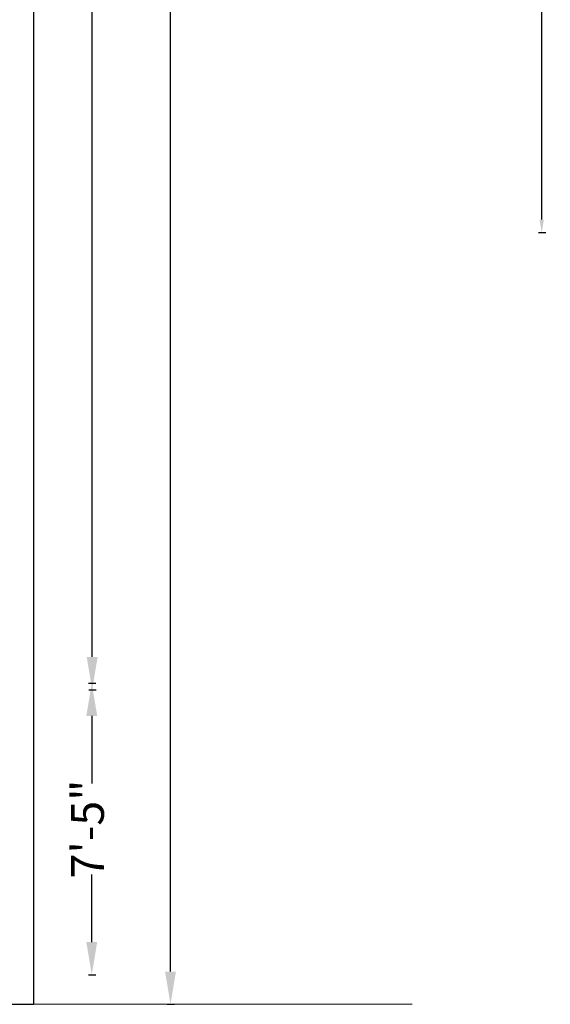
# Model space of a CAD drawing. Units: inches. Extents: x -638 to 186, y -762 to 59.
# Tile 13 of 31: x 24 to 186, y -713 to -413. Entities that reach past the tile are written whole.
import ezdxf

# ---------------------------------------------------------------- set-up
doc = ezdxf.new("R2010")
doc.units = ezdxf.units.IN
for name, color, linetype, lineweight in [('A-ANNO-DIMS', 2, 'Continuous', 18), ('C-PROP', 7, 'Continuous', 25), ('C-ROAD', 7, 'Continuous', 18)]:
    doc.layers.add(name, color=color, linetype=linetype, lineweight=lineweight)
doc.styles.get("Standard").update_dxf_attribs({"font": 'arial.ttf'})
doc.dimstyles.new('ISO-25', dxfattribs={"dimtxt": 4, "dimasz": 4, "dimexe": 1.25, "dimexo": 0.625, "dimtad": 0, "dimlunit": 4, "dimtxsty": 'Standard', "dimcen": 2.5, "dimclrt": 256, "dimadec": 0, "dimazin": 0, "dimtfac": 1, "dimtmove": 0, "dimatfit": 3, "dimfxl": 1, "dimfxlon": 1, "dimarcsym": 0})

# ---------------------------------------------------------------- blocks, each defined once
blk = doc.blocks.new('*D12')
at = {"layer": 'A-ANNO-DIMS', "color": 0, "lineweight": -2, "transparency": 16777216}
for p, q in [((45.29, -615.03), (47.54, -615.03)), ((46.29, -625.03), (46.29, -645.66)), ((46.29, -694.03), (46.29, -673.41)), ((45.29, -704.03), (47.54, -704.03))]:
    blk.add_line(p, q, dxfattribs=at)
at = {"layer": 'A-ANNO-DIMS', "color": 0, "lineweight": 30, "transparency": 16777216}
for points in [[(44.62, -625.03), (47.95, -625.03), (46.29, -615.03)], [(44.62, -694.03), (47.95, -694.03), (46.29, -704.03)]]:
    blk.add_solid(points, dxfattribs=at)
at = {"layer": 'Defpoints', "color": 0, "lineweight": 30, "transparency": 16777216}
for p in [(20.08, -615.03), (20.08, -704.03), (46.29, -704.03)]:
    blk.add_point(p, dxfattribs=at)
at = {"layer": 'A-ANNO-DIMS', "color": 0, "transparency": 16777216, "insert": (46.29, -659.53), "char_height": 10, "attachment_point": 5, "rotation": 90}
blk.add_mtext('7\'-5"', dxfattribs=at)
blk = doc.blocks.new('*D14')
at = {"layer": 'A-ANNO-DIMS', "color": 0, "lineweight": -2, "transparency": 16777216}
for p, q in [((45.41, -42.03), (47.66, -42.03)), ((46.41, -52.03), (46.41, -307.65)), ((46.41, -607.03), (46.41, -351.42)), ((45.41, -617.03), (47.66, -617.03))]:
    blk.add_line(p, q, dxfattribs=at)
at = {"layer": 'A-ANNO-DIMS', "color": 0, "lineweight": 30, "transparency": 16777216}
for points in [[(44.74, -52.03), (48.08, -52.03), (46.41, -42.03)], [(44.74, -607.03), (48.08, -607.03), (46.41, -617.03)]]:
    blk.add_solid(points, dxfattribs=at)
at = {"layer": 'Defpoints', "color": 0, "lineweight": 30, "transparency": 16777216}
for p in [(10.47, -42.03), (10.47, -617.03), (46.41, -617.03)]:
    blk.add_point(p, dxfattribs=at)
at = {"layer": 'A-ANNO-DIMS', "color": 0, "transparency": 16777216, "insert": (46.41, -329.53), "char_height": 10, "attachment_point": 5, "rotation": 90}
blk.add_mtext('47\'-11"', dxfattribs=at)
blk = doc.blocks.new('*D15')
at = {"layer": 'A-ANNO-DIMS', "color": 0, "lineweight": -2, "transparency": 16777216}
for p, q in [((69.33, -24.03), (71.58, -24.03)), ((70.33, -34.03), (70.33, -350.73)), ((70.33, -703.03), (70.33, -386.33)), ((69.33, -713.03), (71.58, -713.03))]:
    blk.add_line(p, q, dxfattribs=at)
at = {"layer": 'A-ANNO-DIMS', "color": 0, "lineweight": 30, "transparency": 16777216}
for points in [[(68.66, -34.03), (72, -34.03), (70.33, -24.03)], [(68.66, -703.03), (72, -703.03), (70.33, -713.03)]]:
    blk.add_solid(points, dxfattribs=at)
at = {"layer": 'Defpoints', "color": 0, "lineweight": 30, "transparency": 16777216}
for p in [(-24.67, -24.03), (-10.56, -713.03), (70.33, -713.03)]:
    blk.add_point(p, dxfattribs=at)
at = {"layer": 'A-ANNO-DIMS', "color": 0, "transparency": 16777216, "insert": (70.33, -368.53), "char_height": 10, "attachment_point": 5, "rotation": 90}
blk.add_mtext('57\'-5"', dxfattribs=at)
blk = doc.blocks.new('*D38')
at = {"layer": 'A-ANNO-DIMS', "color": 0, "lineweight": -2, "transparency": 16777216}
for p, q in [((182.66, -280.53), (184.91, -280.53)), ((183.66, -284.53), (183.66, -371.73)), ((183.66, -473.53), (183.66, -386.34)), ((182.66, -477.53), (184.91, -477.53))]:
    blk.add_line(p, q, dxfattribs=at)
at = {"layer": 'A-ANNO-DIMS', "color": 0, "lineweight": 30, "transparency": 16777216}
for points in [[(183, -284.53), (184.33, -284.53), (183.66, -280.53)], [(183, -473.53), (184.33, -473.53), (183.66, -477.53)]]:
    blk.add_solid(points, dxfattribs=at)
at = {"layer": 'Defpoints', "color": 0, "lineweight": 30, "transparency": 16777216}
for p in [(-404.53, -280.53), (-404.53, -477.53), (183.66, -477.53)]:
    blk.add_point(p, dxfattribs=at)
at = {"layer": 'A-ANNO-DIMS', "transparency": 16777216, "insert": (183.66, -379.03), "char_height": 4, "attachment_point": 5, "rotation": 90}
blk.add_mtext('16\'-5"', dxfattribs=at)

msp = doc.modelspace()

# ---------------------------------------------------------------- linework, layer by layer
at = {"layer": 'C-PROP'}
for p in [(28.474, -24.033), (-116.044, -713.033)]:
    msp.add_line(p, (28.474, -713.033), dxfattribs=at)
at = {"layer": 'C-ROAD'}
msp.add_line((28.474, -713.033), (144.113, -713.033), dxfattribs=at)

# ---------------------------------------------------------------- dimensions: what is measured, and where the dimension line sits
at = {"layer": 'A-ANNO-DIMS'}
for base, p1, p2, override, picture, middle in [((70.331, -713.033), (-24.669, -24.033), (-10.563, -713.033), {"dimtxt": 10, "dimasz": 10, "dimclrd": 0, "dimclre": 0, "dimclrt": 0}, '*D15', (70.331, -368.533)), ((46.411, -617.033), (10.474, -42.033), (10.474, -617.033), {"dimtxt": 10, "dimasz": 10, "dimclrd": 0, "dimclre": 0, "dimclrt": 0}, '*D14', (46.411, -329.533)), ((183.663, -477.533), (-404.526, -280.533), (-404.526, -477.533), {"dimdec": 1, "dimlfac": 1, "dimrnd": 0, "dimzin": 1, "dimdsep": 46, "dimlunit": 4, "dimfrac": 2}, '*D38', (183.663, -379.033)), ((46.286, -704.033), (20.081, -615.033), (20.081, -704.033), {"dimtxt": 10, "dimasz": 10, "dimclrd": 0, "dimclre": 0, "dimclrt": 0}, '*D12', (46.286, -659.533))]:
    dim = msp.add_linear_dim(base=base, p1=p1, p2=p2, angle=90, dimstyle='ISO-25', override=override, dxfattribs=at)
    dim.commit()
    dim.dimension.update_dxf_attribs({"geometry": picture, "text_midpoint": middle})

doc.saveas('drawing.dxf')
